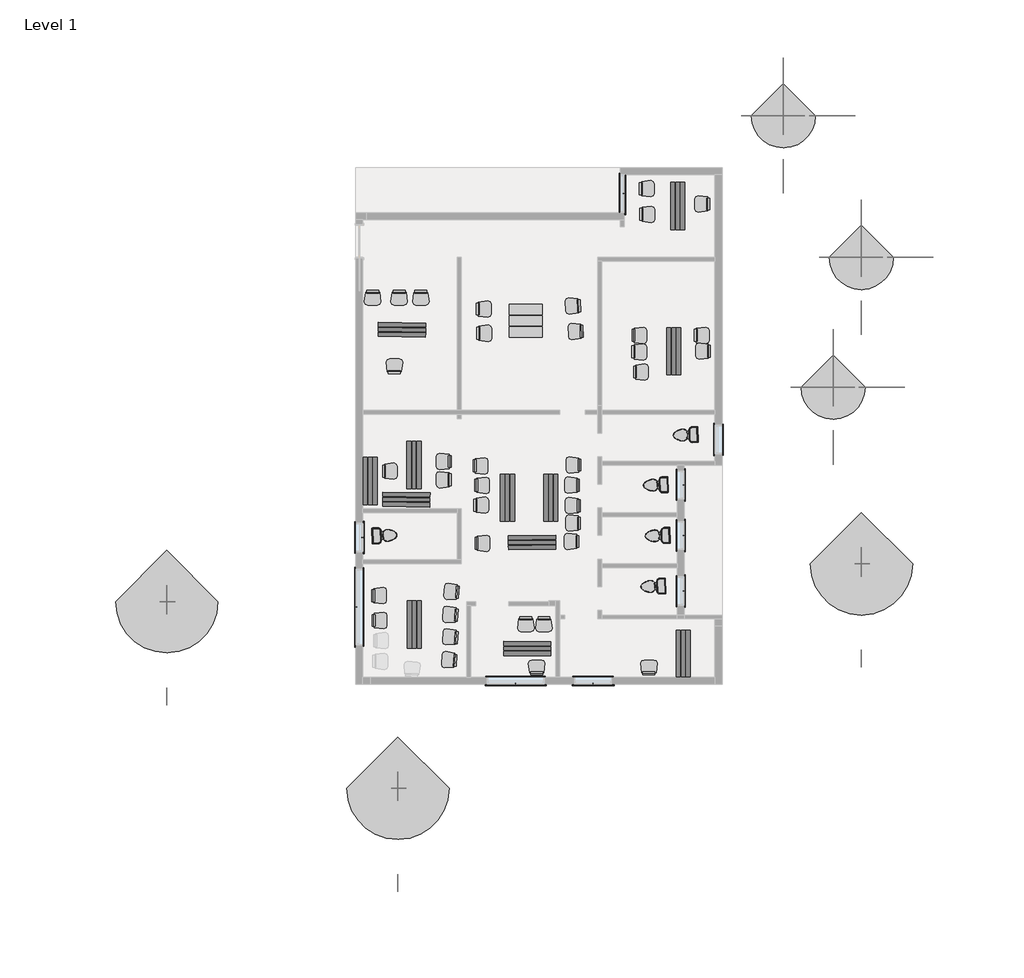
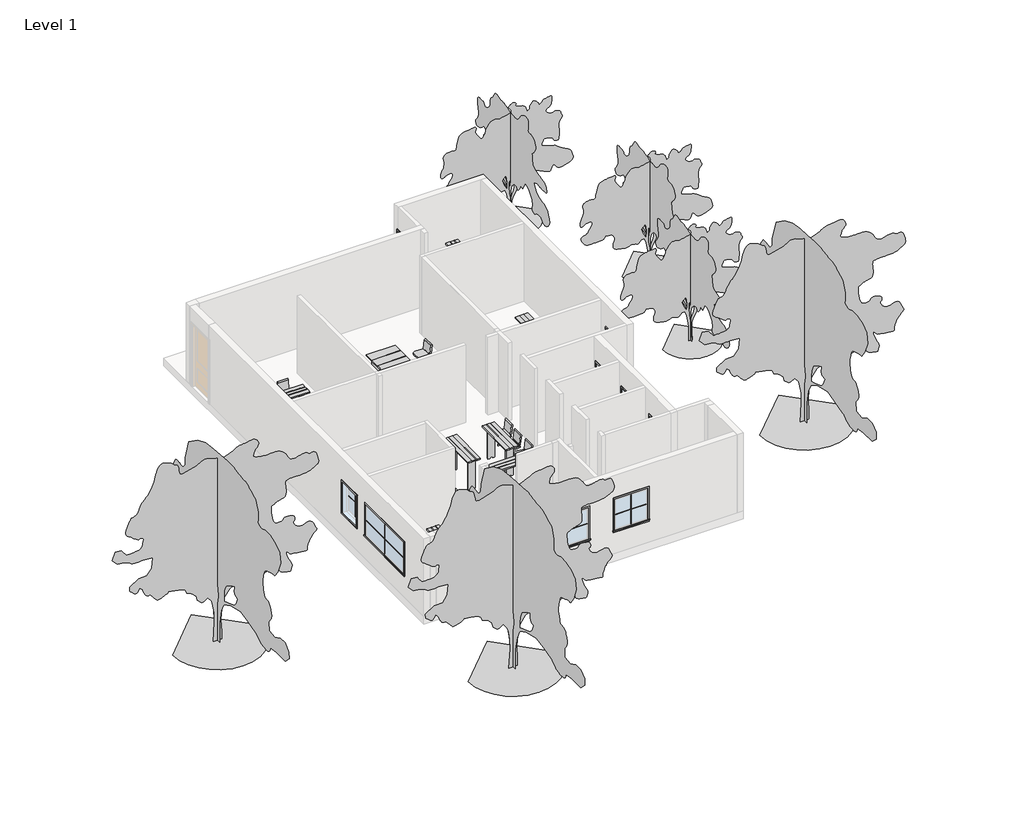
# One storey, part 2 of 2: 51 furniture elements, 27 proxies, 6 geographic elements, 5 flow terminals.
"""IFC4 building model written with IfcOpenShell, lengths in millimetres."""

from ifc_helpers import new_model, si_unit, origin, place, context, project, spatial, transform, mapped, element, save
from components import muntin_pattern_2x2_muntin_pattern_2x2_0b2f62cf, muntin_pattern_2x2_muntin_pattern_2x2_3e35e312, muntin_pattern_2x2_muntin_pattern_2x2_6be186e8, muntin_pattern_2x2_muntin_pattern_2x2_2dc59915, trim_window_exterior_flat_with_sill_e4b28ec3, trim_window_exterior_flat_with_sill_7cfdd449, trim_window_exterior_flat_with_sill_4ebd5beb, trim_window_exterior_flat_with_sill_02d88a07, trim_window_interior_flat_picture_frame_39ff4276, trim_window_interior_flat_picture_frame_f1e0b15b, trim_window_interior_flat_picture_frame_d03d3773, trim_window_interior_flat_picture_frame_03e64d7c, toilet_domestic_3d_toilet_domestic_3d_ba6479b0, toilet_domestic_3d_toilet_domestic_3d_30431060, furniture_f7008d8d, furniture_92cb3fd8, chair_desk_chair_desk_7ad88740, chair_desk_chair_desk_f6d25cbe, rpc_tree_deciduous_blue_berry_elder_15_a2d70376, rpc_tree_deciduous_hawthorn_25_a438f522

model = new_model("IFC4")

# Units and contexts
model_context = context("Model", 3, world=origin())
ifc_project = project(units=[si_unit("LENGTHUNIT", "METRE", prefix="MILLI")], contexts=[model_context])

# Site, building, storey
site = spatial("IfcSite", under=ifc_project)
building = spatial("IfcBuilding", under=site)
storey = spatial("IfcBuildingStorey", under=building, Name="Level 1", Elevation=0.0)

# Proxies
placement = place(None, origin())
muntin_pattern_2x2_muntin_pattern_2x2_shape = muntin_pattern_2x2_muntin_pattern_2x2_0b2f62cf(model_context)
element("IfcBuildingElementProxy", 1, Name="Muntin Pattern_2x2 : Muntin Pattern_2x2", ObjectType="Muntin Pattern_2x2 : Muntin Pattern_2x2", at=placement, inside=storey, context=model_context, shape_type="MappedRepresentation", body=[
    mapped(muntin_pattern_2x2_muntin_pattern_2x2_shape, transform((11852.275, 18726.15, 952.5), x_axis=(0.0, 1.0, 0.0), y_axis=(-1.0, 0.0, 0.0), z_axis=(0.0, 0.0, 1.0))),
])
element("IfcBuildingElementProxy", 2, Name="Muntin Pattern_2x2 : Muntin Pattern_2x2", ObjectType="Muntin Pattern_2x2 : Muntin Pattern_2x2", at=placement, inside=storey, context=model_context, shape_type="MappedRepresentation", body=[
    mapped(muntin_pattern_2x2_muntin_pattern_2x2_shape, transform((12861.925, 20186.0468811, 952.5), x_axis=(0.0, -1.0, 0.0), y_axis=(1.0, 0.0, 0.0), z_axis=(0.0, 0.0, 1.0))),
])
element("IfcBuildingElementProxy", 3, Name="Muntin Pattern_2x2 : Muntin Pattern_2x2", ObjectType="Muntin Pattern_2x2 : Muntin Pattern_2x2", at=placement, inside=storey, context=model_context, shape_type="MappedRepresentation", body=[
    mapped(muntin_pattern_2x2_muntin_pattern_2x2_shape, transform((1489.075, 17029.3631818, 952.5), x_axis=(0.0, 1.0, 0.0), y_axis=(-1.0, 0.0, 0.0), z_axis=(0.0, 0.0, 1.0))),
])
element("IfcBuildingElementProxy", 4, Name="Muntin Pattern_2x2 : Muntin Pattern_2x2", ObjectType="Muntin Pattern_2x2 : Muntin Pattern_2x2", at=placement, inside=storey, context=model_context, shape_type="MappedRepresentation", body=[
    mapped(muntin_pattern_2x2_muntin_pattern_2x2_shape, transform((11852.275, 15299.8267416, 952.5), x_axis=(0.0, 1.0, 0.0), y_axis=(-1.0, 0.0, 0.0), z_axis=(0.0, 0.0, 1.0))),
])
element("IfcBuildingElementProxy", 5, Name="Muntin Pattern_2x2 : Muntin Pattern_2x2", ObjectType="Muntin Pattern_2x2 : Muntin Pattern_2x2", at=placement, inside=storey, context=model_context, shape_type="MappedRepresentation", body=[
    mapped(muntin_pattern_2x2_muntin_pattern_2x2_shape, transform((11852.275, 17092.3067598, 952.5), x_axis=(0.0, 1.0, 0.0), y_axis=(-1.0, 0.0, 0.0), z_axis=(0.0, 0.0, 1.0))),
])
muntin_pattern_2x2_muntin_pattern_2x2_2_shape = muntin_pattern_2x2_muntin_pattern_2x2_3e35e312(model_context)
element("IfcBuildingElementProxy", 6, Name="Muntin Pattern_2x2 : Muntin Pattern_2x2", ObjectType="Muntin Pattern_2x2 : Muntin Pattern_2x2", at=placement, inside=storey, context=model_context, shape_type="MappedRepresentation", body=[
    mapped(muntin_pattern_2x2_muntin_pattern_2x2_2_shape, transform((9921.875, 28117.8, 952.5), x_axis=(0.0, 1.0, 0.0), y_axis=(-1.0, 0.0, 0.0), z_axis=(0.0, 0.0, 1.0))),
])
element("IfcBuildingElementProxy", 7, Name="Muntin Pattern_2x2 : Muntin Pattern_2x2", ObjectType="Muntin Pattern_2x2 : Muntin Pattern_2x2", at=placement, inside=storey, context=model_context, shape_type="MappedRepresentation", body=[
    mapped(muntin_pattern_2x2_muntin_pattern_2x2_2_shape, transform((8921.75, 12303.125, 952.5), x_axis=(1.0, 0.0, 0.0), y_axis=(0.0, 1.0, 0.0), z_axis=(0.0, 0.0, 1.0))),
])
muntin_pattern_2x2_muntin_pattern_2x2_3_shape = muntin_pattern_2x2_muntin_pattern_2x2_6be186e8(model_context)
element("IfcBuildingElementProxy", 8, Name="Muntin Pattern_2x2 : Muntin Pattern_2x2", ObjectType="Muntin Pattern_2x2 : Muntin Pattern_2x2", at=placement, inside=storey, context=model_context, shape_type="MappedRepresentation", body=[
    mapped(muntin_pattern_2x2_muntin_pattern_2x2_3_shape, transform((1279.525, 14783.4980131, 952.5), x_axis=(0.0, -1.0, 0.0), y_axis=(1.0, 0.0, 0.0), z_axis=(0.0, 0.0, 1.0))),
])
muntin_pattern_2x2_muntin_pattern_2x2_4_shape = muntin_pattern_2x2_muntin_pattern_2x2_2dc59915(model_context)
element("IfcBuildingElementProxy", 9, Name="Muntin Pattern_2x2 : Muntin Pattern_2x2", ObjectType="Muntin Pattern_2x2 : Muntin Pattern_2x2", at=placement, inside=storey, context=model_context, shape_type="MappedRepresentation", body=[
    mapped(muntin_pattern_2x2_muntin_pattern_2x2_4_shape, transform((6426.2, 12303.125, 952.5), x_axis=(1.0, 0.0, 0.0), y_axis=(0.0, 1.0, 0.0), z_axis=(0.0, 0.0, 1.0))),
])
trim_window_exterior_flat_with_sill_shape = trim_window_exterior_flat_with_sill_e4b28ec3(model_context)
element("IfcBuildingElementProxy", 10, Name="Trim-Window-Exterior-Flat : with Sill", ObjectType="Trim-Window-Exterior-Flat : with Sill", at=placement, inside=storey, context=model_context, shape_type="MappedRepresentation", body=[
    mapped(trim_window_exterior_flat_with_sill_shape, transform((11861.8, 18726.15, 2133.6), x_axis=(0.0, 1.0, 0.0), y_axis=(0.0, 0.0, 1.0), z_axis=(1.0, 0.0, 0.0))),
])
element("IfcBuildingElementProxy", 11, Name="Trim-Window-Exterior-Flat : with Sill", ObjectType="Trim-Window-Exterior-Flat : with Sill", at=placement, inside=storey, context=model_context, shape_type="MappedRepresentation", body=[
    mapped(trim_window_exterior_flat_with_sill_shape, transform((12852.4, 20186.0468811, 2133.6), x_axis=(0.0, -1.0, 0.0), y_axis=(0.0, 0.0, 1.0), z_axis=(-1.0, 0.0, 0.0))),
])
element("IfcBuildingElementProxy", 12, Name="Trim-Window-Exterior-Flat : with Sill", ObjectType="Trim-Window-Exterior-Flat : with Sill", at=placement, inside=storey, context=model_context, shape_type="MappedRepresentation", body=[
    mapped(trim_window_exterior_flat_with_sill_shape, transform((1498.6, 17029.3631818, 2133.6), x_axis=(0.0, 1.0, 0.0), y_axis=(0.0, 0.0, 1.0), z_axis=(1.0, 0.0, 0.0))),
])
element("IfcBuildingElementProxy", 13, Name="Trim-Window-Exterior-Flat : with Sill", ObjectType="Trim-Window-Exterior-Flat : with Sill", at=placement, inside=storey, context=model_context, shape_type="MappedRepresentation", body=[
    mapped(trim_window_exterior_flat_with_sill_shape, transform((11861.8, 15299.8267416, 2133.6), x_axis=(0.0, 1.0, 0.0), y_axis=(0.0, 0.0, 1.0), z_axis=(1.0, 0.0, 0.0))),
])
element("IfcBuildingElementProxy", 14, Name="Trim-Window-Exterior-Flat : with Sill", ObjectType="Trim-Window-Exterior-Flat : with Sill", at=placement, inside=storey, context=model_context, shape_type="MappedRepresentation", body=[
    mapped(trim_window_exterior_flat_with_sill_shape, transform((11861.8, 17092.3067598, 2133.6), x_axis=(0.0, 1.0, 0.0), y_axis=(0.0, 0.0, 1.0), z_axis=(1.0, 0.0, 0.0))),
])
trim_window_exterior_flat_with_sill_2_shape = trim_window_exterior_flat_with_sill_7cfdd449(model_context)
element("IfcBuildingElementProxy", 15, Name="Trim-Window-Exterior-Flat : with Sill", ObjectType="Trim-Window-Exterior-Flat : with Sill", at=placement, inside=storey, context=model_context, shape_type="MappedRepresentation", body=[
    mapped(trim_window_exterior_flat_with_sill_2_shape, transform((9931.4, 28117.8, 2133.6), x_axis=(0.0, 1.0, 0.0), y_axis=(0.0, 0.0, 1.0), z_axis=(1.0, 0.0, 0.0))),
])
element("IfcBuildingElementProxy", 16, Name="Trim-Window-Exterior-Flat : with Sill", ObjectType="Trim-Window-Exterior-Flat : with Sill", at=placement, inside=storey, context=model_context, shape_type="MappedRepresentation", body=[
    mapped(trim_window_exterior_flat_with_sill_2_shape, transform((8921.75, 12293.6, 2133.6), x_axis=(1.0, 0.0, 0.0), y_axis=(0.0, 0.0, 1.0), z_axis=(0.0, -1.0, 0.0))),
])
trim_window_exterior_flat_with_sill_3_shape = trim_window_exterior_flat_with_sill_4ebd5beb(model_context)
element("IfcBuildingElementProxy", 17, Name="Trim-Window-Exterior-Flat : with Sill", ObjectType="Trim-Window-Exterior-Flat : with Sill", at=placement, inside=storey, context=model_context, shape_type="MappedRepresentation", body=[
    mapped(trim_window_exterior_flat_with_sill_3_shape, transform((1270.0, 14783.4980131, 2133.6), x_axis=(0.0, -1.0, 0.0), y_axis=(0.0, 0.0, 1.0), z_axis=(-1.0, 0.0, 0.0))),
])
trim_window_exterior_flat_with_sill_4_shape = trim_window_exterior_flat_with_sill_02d88a07(model_context)
element("IfcBuildingElementProxy", 18, Name="Trim-Window-Exterior-Flat : with Sill", ObjectType="Trim-Window-Exterior-Flat : with Sill", at=placement, inside=storey, context=model_context, shape_type="MappedRepresentation", body=[
    mapped(trim_window_exterior_flat_with_sill_4_shape, transform((6426.2, 12293.6, 2133.6), x_axis=(1.0, 0.0, 0.0), y_axis=(0.0, 0.0, 1.0), z_axis=(0.0, -1.0, 0.0))),
])
trim_window_interior_flat_picture_frame_shape = trim_window_interior_flat_picture_frame_39ff4276(model_context)
element("IfcBuildingElementProxy", 19, Name="Trim-Window-Interior-Flat : Picture Frame", ObjectType="Trim-Window-Interior-Flat : Picture Frame", at=placement, inside=storey, context=model_context, shape_type="MappedRepresentation", body=[
    mapped(trim_window_interior_flat_picture_frame_shape, transform((11633.2, 18726.15, 2133.6), x_axis=(0.0, -1.0, 0.0), y_axis=(0.0, 0.0, 1.0), z_axis=(-1.0, 0.0, 0.0))),
])
element("IfcBuildingElementProxy", 20, Name="Trim-Window-Interior-Flat : Picture Frame", ObjectType="Trim-Window-Interior-Flat : Picture Frame", at=placement, inside=storey, context=model_context, shape_type="MappedRepresentation", body=[
    mapped(trim_window_interior_flat_picture_frame_shape, transform((13081.0, 20186.0468811, 2133.6), x_axis=(0.0, 1.0, 0.0), y_axis=(0.0, 0.0, 1.0), z_axis=(1.0, 0.0, 0.0))),
])
element("IfcBuildingElementProxy", 21, Name="Trim-Window-Interior-Flat : Picture Frame", ObjectType="Trim-Window-Interior-Flat : Picture Frame", at=placement, inside=storey, context=model_context, shape_type="MappedRepresentation", body=[
    mapped(trim_window_interior_flat_picture_frame_shape, transform((1270.0, 17029.3631818, 2133.6), x_axis=(0.0, -1.0, 0.0), y_axis=(0.0, 0.0, 1.0), z_axis=(-1.0, 0.0, 0.0))),
])
element("IfcBuildingElementProxy", 22, Name="Trim-Window-Interior-Flat : Picture Frame", ObjectType="Trim-Window-Interior-Flat : Picture Frame", at=placement, inside=storey, context=model_context, shape_type="MappedRepresentation", body=[
    mapped(trim_window_interior_flat_picture_frame_shape, transform((11633.2, 15299.8267416, 2133.6), x_axis=(0.0, -1.0, 0.0), y_axis=(0.0, 0.0, 1.0), z_axis=(-1.0, 0.0, 0.0))),
])
element("IfcBuildingElementProxy", 23, Name="Trim-Window-Interior-Flat : Picture Frame", ObjectType="Trim-Window-Interior-Flat : Picture Frame", at=placement, inside=storey, context=model_context, shape_type="MappedRepresentation", body=[
    mapped(trim_window_interior_flat_picture_frame_shape, transform((11633.2, 17092.3067598, 2133.6), x_axis=(0.0, -1.0, 0.0), y_axis=(0.0, 0.0, 1.0), z_axis=(-1.0, 0.0, 0.0))),
])
trim_window_interior_flat_picture_frame_2_shape = trim_window_interior_flat_picture_frame_f1e0b15b(model_context)
element("IfcBuildingElementProxy", 24, Name="Trim-Window-Interior-Flat : Picture Frame", ObjectType="Trim-Window-Interior-Flat : Picture Frame", at=placement, inside=storey, context=model_context, shape_type="MappedRepresentation", body=[
    mapped(trim_window_interior_flat_picture_frame_2_shape, transform((9804.4, 28117.8, 2133.6), x_axis=(0.0, -1.0, 0.0), y_axis=(0.0, 0.0, 1.0), z_axis=(-1.0, 0.0, 0.0))),
])
element("IfcBuildingElementProxy", 25, Name="Trim-Window-Interior-Flat : Picture Frame", ObjectType="Trim-Window-Interior-Flat : Picture Frame", at=placement, inside=storey, context=model_context, shape_type="MappedRepresentation", body=[
    mapped(trim_window_interior_flat_picture_frame_2_shape, transform((8921.75, 12522.2, 2133.6), x_axis=(-1.0, 0.0, 0.0), y_axis=(0.0, 0.0, 1.0), z_axis=(0.0, 1.0, 0.0))),
])
trim_window_interior_flat_picture_frame_3_shape = trim_window_interior_flat_picture_frame_d03d3773(model_context)
element("IfcBuildingElementProxy", 26, Name="Trim-Window-Interior-Flat : Picture Frame", ObjectType="Trim-Window-Interior-Flat : Picture Frame", at=placement, inside=storey, context=model_context, shape_type="MappedRepresentation", body=[
    mapped(trim_window_interior_flat_picture_frame_3_shape, transform((1498.6, 14783.4980131, 2133.6), x_axis=(0.0, 1.0, 0.0), y_axis=(0.0, 0.0, 1.0), z_axis=(1.0, 0.0, 0.0))),
])
trim_window_interior_flat_picture_frame_4_shape = trim_window_interior_flat_picture_frame_03e64d7c(model_context)
element("IfcBuildingElementProxy", 27, Name="Trim-Window-Interior-Flat : Picture Frame", ObjectType="Trim-Window-Interior-Flat : Picture Frame", at=placement, inside=storey, context=model_context, shape_type="MappedRepresentation", body=[
    mapped(trim_window_interior_flat_picture_frame_4_shape, transform((6426.2, 12522.2, 2133.6), x_axis=(-1.0, 0.0, 0.0), y_axis=(0.0, 0.0, 1.0), z_axis=(0.0, 1.0, 0.0))),
])

# Flow terminals
toilet_domestic_3d_toilet_domestic_3d_shape = toilet_domestic_3d_toilet_domestic_3d_ba6479b0(model_context)
toilet_domestic_3d_toilet_domestic_3d_2_shape = toilet_domestic_3d_toilet_domestic_3d_30431060(model_context)
element("IfcFlowTerminal", 28, ObjectType="Toilet-Domestic-3D : Toilet-Domestic-3D", at=placement, inside=storey, context=model_context, shape_type="MappedRepresentation", body=[
    mapped(toilet_domestic_3d_toilet_domestic_3d_shape, transform((11812.081271, 20333.332001, 0.0), x_axis=(0.0355411275689283, -0.9993682145491367, 0.0), y_axis=(0.9993682145491367, 0.0355411275689283, 0.0), z_axis=(0.0, 0.0, 1.0))),
    mapped(toilet_domestic_3d_toilet_domestic_3d_2_shape, transform((11812.081271, 20333.332001, 0.0), x_axis=(0.0355411275689283, -0.9993682145491367, 0.0), y_axis=(0.9993682145491367, 0.0355411275689283, 0.0), z_axis=(0.0, 0.0, 1.0))),
])
element("IfcFlowTerminal", 29, ObjectType="Toilet-Domestic-3D : Toilet-Domestic-3D", at=placement, inside=storey, context=model_context, shape_type="MappedRepresentation", body=[
    mapped(toilet_domestic_3d_toilet_domestic_3d_shape, transform((10850.8877462, 18719.2515392, 0.0), x_axis=(0.03554112756892187, -0.9993682145491369, 0.0), y_axis=(0.9993682145491369, 0.03554112756892187, 0.0), z_axis=(0.0, 0.0, 1.0))),
    mapped(toilet_domestic_3d_toilet_domestic_3d_2_shape, transform((10850.8877462, 18719.2515392, 0.0), x_axis=(0.03554112756892187, -0.9993682145491369, 0.0), y_axis=(0.9993682145491369, 0.03554112756892187, 0.0), z_axis=(0.0, 0.0, 1.0))),
])
element("IfcFlowTerminal", 30, ObjectType="Toilet-Domestic-3D : Toilet-Domestic-3D", at=placement, inside=storey, context=model_context, shape_type="MappedRepresentation", body=[
    mapped(toilet_domestic_3d_toilet_domestic_3d_shape, transform((10908.9901447, 17085.4910432, 0.0), x_axis=(0.03554112756892187, -0.9993682145491369, 0.0), y_axis=(0.9993682145491369, 0.03554112756892187, 0.0), z_axis=(0.0, 0.0, 1.0))),
    mapped(toilet_domestic_3d_toilet_domestic_3d_2_shape, transform((10908.9901447, 17085.4910432, 0.0), x_axis=(0.03554112756892187, -0.9993682145491369, 0.0), y_axis=(0.9993682145491369, 0.03554112756892187, 0.0), z_axis=(0.0, 0.0, 1.0))),
])
element("IfcFlowTerminal", 31, ObjectType="Toilet-Domestic-3D : Toilet-Domestic-3D", at=placement, inside=storey, context=model_context, shape_type="MappedRepresentation", body=[
    mapped(toilet_domestic_3d_toilet_domestic_3d_shape, transform((10770.2616437, 15450.0084658, 0.0), x_axis=(0.03554112756892187, -0.9993682145491369, 0.0), y_axis=(0.9993682145491369, 0.03554112756892187, 0.0), z_axis=(0.0, 0.0, 1.0))),
    mapped(toilet_domestic_3d_toilet_domestic_3d_2_shape, transform((10770.2616437, 15450.0084658, 0.0), x_axis=(0.03554112756892187, -0.9993682145491369, 0.0), y_axis=(0.9993682145491369, 0.03554112756892187, 0.0), z_axis=(0.0, 0.0, 1.0))),
])
element("IfcFlowTerminal", 32, ObjectType="Toilet-Domestic-3D : Toilet-Domestic-3D", at=placement, inside=storey, context=model_context, shape_type="MappedRepresentation", body=[
    mapped(toilet_domestic_3d_toilet_domestic_3d_shape, transform((2292.7062712, 17095.9305022, 0.0), x_axis=(-0.03572734203544766, 0.9993615747221234, 0.0), y_axis=(-0.9993615747221234, -0.03572734203544766, 0.0), z_axis=(0.0, 0.0, 1.0))),
    mapped(toilet_domestic_3d_toilet_domestic_3d_2_shape, transform((2292.7062712, 17095.9305022, 0.0), x_axis=(-0.03572734203544766, 0.9993615747221234, 0.0), y_axis=(-0.9993615747221234, -0.03572734203544766, 0.0), z_axis=(0.0, 0.0, 1.0))),
])

# Furniture
furniture_shape = furniture_f7008d8d(model_context)
element("IfcFurniture", 33, ObjectType="Bench-Locker Room : 48\" x 18\" x 14\"", at=placement, inside=storey, context=model_context, shape_type="MappedRepresentation", body=[
    mapped(furniture_shape, transform((2974.0575649, 14379.3147541, 0.0), x_axis=(0.0, 1.0, 0.0), y_axis=(-1.0, 0.0, 0.0), z_axis=(0.0, 0.0, 1.0))),
])
element("IfcFurniture", 34, ObjectType="Bench-Locker Room : 48\" x 18\" x 14\"", at=placement, inside=storey, context=model_context, shape_type="MappedRepresentation", body=[
    mapped(furniture_shape, transform((2917.3364211, 23908.3455859, 0.0), x_axis=(0.9998480894786371, -0.017429801086626003, 0.0), y_axis=(0.017429801086626003, 0.9998480894786371, 0.0), z_axis=(0.0, 0.0, 1.0))),
])
element("IfcFurniture", 35, ObjectType="Bench-Locker Room : 48\" x 18\" x 14\"", at=placement, inside=storey, context=model_context, shape_type="MappedRepresentation", body=[
    mapped(furniture_shape, transform((11830.2076457, 27568.7581913, 0.0), x_axis=(0.0, -1.0, 0.0), y_axis=(1.0, 0.0, 0.0), z_axis=(0.0, 0.0, 1.0))),
])
element("IfcFurniture", 36, ObjectType="Bench-Locker Room : 48\" x 18\" x 14\"", at=placement, inside=storey, context=model_context, shape_type="MappedRepresentation", body=[
    mapped(furniture_shape, transform((11704.0646955, 22884.2865861, 0.0), x_axis=(0.0, -1.0, 0.0), y_axis=(1.0, 0.0, 0.0), z_axis=(0.0, 0.0, 1.0))),
])
element("IfcFurniture", 37, ObjectType="Bench-Locker Room : 48\" x 18\" x 14\"", at=placement, inside=storey, context=model_context, shape_type="MappedRepresentation", body=[
    mapped(furniture_shape, transform((5979.6841277, 18462.9611479, 0.0), x_axis=(0.0, 1.0, 0.0), y_axis=(-1.0, 0.0, 0.0), z_axis=(0.0, 0.0, 1.0))),
])
element("IfcFurniture", 38, ObjectType="Bench-Locker Room : 48\" x 18\" x 14\"", at=placement, inside=storey, context=model_context, shape_type="MappedRepresentation", body=[
    mapped(furniture_shape, transform((6801.6796201, 16686.4490944, 0.0), x_axis=(-0.9999200930744279, -0.012641497776273655, 0.0), y_axis=(0.012641497776273655, -0.9999200930744279, 0.0), z_axis=(0.0, 0.0, 1.0))),
])
element("IfcFurniture", 39, ObjectType="Bench-Locker Room : 48\" x 18\" x 14\"", at=placement, inside=storey, context=model_context, shape_type="MappedRepresentation", body=[
    mapped(furniture_shape, transform((1553.7196201, 19010.7185302, 0.0), x_axis=(0.0, 1.0, 0.0), y_axis=(-1.0, 0.0, 0.0), z_axis=(0.0, 0.0, 1.0))),
])
element("IfcFurniture", 40, ObjectType="Bench-Locker Room : 48\" x 18\" x 14\"", at=placement, inside=storey, context=model_context, shape_type="MappedRepresentation", body=[
    mapped(furniture_shape, transform((12008.8646955, 13125.8549349, 0.0), x_axis=(0.0, -1.0, 0.0), y_axis=(1.0, 0.0, 0.0), z_axis=(0.0, 0.0, 1.0))),
])
element("IfcFurniture", 41, ObjectType="Bench-Locker Room : 48\" x 18\" x 14\"", at=placement, inside=storey, context=model_context, shape_type="MappedRepresentation", body=[
    mapped(furniture_shape, transform((6640.7852173, 13265.3501596, 0.0), x_axis=(-0.9999884249581985, 0.004811439454202483, 0.0), y_axis=(-0.004811439454202483, -0.9999884249581985, 0.0), z_axis=(0.0, 0.0, 1.0))),
])
element("IfcFurniture", 42, ObjectType="Bench-Locker Room : 48\" x 18\" x 14\"", at=placement, inside=storey, context=model_context, shape_type="MappedRepresentation", body=[
    mapped(furniture_shape, transform((3055.5684722, 18429.963506, 0.0), x_axis=(0.9998480894786371, -0.017429801086626003, 0.0), y_axis=(0.017429801086626003, 0.9998480894786371, 0.0), z_axis=(0.0, 0.0, 1.0))),
])
element("IfcFurniture", 43, ObjectType="Bench-Locker Room : 48\" x 18\" x 14\"", at=placement, inside=storey, context=model_context, shape_type="MappedRepresentation", body=[
    mapped(furniture_shape, transform((7381.3152378, 18462.9611479, 0.0), x_axis=(0.0, 1.0, 0.0), y_axis=(-1.0, 0.0, 0.0), z_axis=(0.0, 0.0, 1.0))),
])
element("IfcFurniture", 44, ObjectType="Bench-Locker Room : 48\" x 18\" x 14\"", at=placement, inside=storey, context=model_context, shape_type="MappedRepresentation", body=[
    mapped(furniture_shape, transform((2964.6454164, 19518.8936677, 0.0), x_axis=(0.0, 1.0, 0.0), y_axis=(-1.0, 0.0, 0.0), z_axis=(0.0, 0.0, 1.0))),
])
furniture_2_shape = furniture_92cb3fd8(model_context)
element("IfcFurniture", 45, ObjectType="Bench-Locker Room : 48\" x 18\" x 18\"", at=placement, inside=storey, context=model_context, shape_type="MappedRepresentation", body=[
    mapped(furniture_2_shape, transform((6908.1087006, 24204.188932, 0.0), x_axis=(1.0, 0.0, 0.0), y_axis=(0.0, 1.0, 0.0), z_axis=(0.0, 0.0, 1.0))),
])
chair_desk_chair_desk_shape = chair_desk_chair_desk_7ad88740(model_context)
element("IfcFurniture", 46, ObjectType="Chair-Desk : Chair-Desk", at=placement, inside=storey, context=model_context, shape_type="MappedRepresentation", body=[
    mapped(chair_desk_chair_desk_shape, transform((8397.3520149, 16903.7, 0.0), x_axis=(0.0, 1.0, 0.0), y_axis=(-1.0, 0.0, 0.0), z_axis=(0.0, 0.0, 1.0))),
])
element("IfcFurniture", 47, ObjectType="Chair-Desk : Chair-Desk", at=placement, inside=storey, context=model_context, shape_type="MappedRepresentation", body=[
    mapped(chair_desk_chair_desk_shape, transform((8444.7345696, 17494.2878949, 0.0), x_axis=(0.0, 1.0, 0.0), y_axis=(-1.0, 0.0, 0.0), z_axis=(0.0, 0.0, 1.0))),
])
element("IfcFurniture", 48, ObjectType="Chair-Desk : Chair-Desk", at=placement, inside=storey, context=model_context, shape_type="MappedRepresentation", body=[
    mapped(chair_desk_chair_desk_shape, transform((8438.3933452, 18054.041753, 0.0), x_axis=(0.0, 1.0, 0.0), y_axis=(-1.0, 0.0, 0.0), z_axis=(0.0, 0.0, 1.0))),
])
element("IfcFurniture", 49, ObjectType="Chair-Desk : Chair-Desk", at=placement, inside=storey, context=model_context, shape_type="MappedRepresentation", body=[
    mapped(chair_desk_chair_desk_shape, transform((4278.1176051, 19481.8, 0.0), x_axis=(0.0, 1.0, 0.0), y_axis=(-1.0, 0.0, 0.0), z_axis=(0.0, 0.0, 1.0))),
])
element("IfcFurniture", 50, ObjectType="Chair-Desk : Chair-Desk", at=placement, inside=storey, context=model_context, shape_type="MappedRepresentation", body=[
    mapped(chair_desk_chair_desk_shape, transform((4275.5800785, 18890.7524599, 0.0), x_axis=(0.0, 1.0, 0.0), y_axis=(-1.0, 0.0, 0.0), z_axis=(0.0, 0.0, 1.0))),
])
element("IfcFurniture", 51, ObjectType="Chair-Desk : Chair-Desk", at=placement, inside=storey, context=model_context, shape_type="MappedRepresentation", body=[
    mapped(chair_desk_chair_desk_shape, transform((8410.2496775, 18715.0954423, 0.0), x_axis=(0.0, 1.0, 0.0), y_axis=(-1.0, 0.0, 0.0), z_axis=(0.0, 0.0, 1.0))),
])
element("IfcFurniture", 52, ObjectType="Chair-Desk : Chair-Desk", at=placement, inside=storey, context=model_context, shape_type="MappedRepresentation", body=[
    mapped(chair_desk_chair_desk_shape, transform((2197.4822905, 19168.4618696, 0.0), x_axis=(0.0, -1.0, 0.0), y_axis=(1.0, 0.0, 0.0), z_axis=(0.0, 0.0, 1.0))),
])
element("IfcFurniture", 53, ObjectType="Chair-Desk : Chair-Desk", at=placement, inside=storey, context=model_context, shape_type="MappedRepresentation", body=[
    mapped(chair_desk_chair_desk_shape, transform((5125.0631491, 19335.7449431, 0.0), x_axis=(0.0, -1.0, 0.0), y_axis=(1.0, 0.0, 0.0), z_axis=(0.0, 0.0, 1.0))),
])
element("IfcFurniture", 54, ObjectType="Chair-Desk : Chair-Desk", at=placement, inside=storey, context=model_context, shape_type="MappedRepresentation", body=[
    mapped(chair_desk_chair_desk_shape, transform((5173.5648431, 18713.4149099, 0.0), x_axis=(0.0, -1.0, 0.0), y_axis=(1.0, 0.0, 0.0), z_axis=(0.0, 0.0, 1.0))),
])
element("IfcFurniture", 55, ObjectType="Chair-Desk : Chair-Desk", at=placement, inside=storey, context=model_context, shape_type="MappedRepresentation", body=[
    mapped(chair_desk_chair_desk_shape, transform((5146.5403146, 18072.1432431, 0.0), x_axis=(0.0, -1.0, 0.0), y_axis=(1.0, 0.0, 0.0), z_axis=(0.0, 0.0, 1.0))),
])
element("IfcFurniture", 56, ObjectType="Chair-Desk : Chair-Desk", at=placement, inside=storey, context=model_context, shape_type="MappedRepresentation", body=[
    mapped(chair_desk_chair_desk_shape, transform((12256.0694835, 23545.9420373, 0.0), x_axis=(0.0, -1.0, 0.0), y_axis=(1.0, 0.0, 0.0), z_axis=(0.0, 0.0, 1.0))),
])
element("IfcFurniture", 57, ObjectType="Chair-Desk : Chair-Desk", at=placement, inside=storey, context=model_context, shape_type="MappedRepresentation", body=[
    mapped(chair_desk_chair_desk_shape, transform((5187.5816449, 16839.2593518, 0.0), x_axis=(0.0, -1.0, 0.0), y_axis=(1.0, 0.0, 0.0), z_axis=(0.0, 0.0, 1.0))),
])
element("IfcFurniture", 58, ObjectType="Chair-Desk : Chair-Desk", at=placement, inside=storey, context=model_context, shape_type="MappedRepresentation", body=[
    mapped(chair_desk_chair_desk_shape, transform((1811.6036816, 24933.2977629, 0.0), x_axis=(-1.0, 0.0, 0.0), y_axis=(0.0, -1.0, 0.0), z_axis=(0.0, 0.0, 1.0))),
])
element("IfcFurniture", 59, ObjectType="Chair-Desk : Chair-Desk", at=placement, inside=storey, context=model_context, shape_type="MappedRepresentation", body=[
    mapped(chair_desk_chair_desk_shape, transform((2665.4699803, 24933.2977629, 0.0), x_axis=(-1.0, 0.0, 0.0), y_axis=(0.0, -1.0, 0.0), z_axis=(0.0, 0.0, 1.0))),
])
element("IfcFurniture", 60, ObjectType="Chair-Desk : Chair-Desk", at=placement, inside=storey, context=model_context, shape_type="MappedRepresentation", body=[
    mapped(chair_desk_chair_desk_shape, transform((3366.8585021, 24931.0160368, 0.0), x_axis=(-1.0, 0.0, 0.0), y_axis=(0.0, -1.0, 0.0), z_axis=(0.0, 0.0, 1.0))),
])
element("IfcFurniture", 61, ObjectType="Chair-Desk : Chair-Desk", at=placement, inside=storey, context=model_context, shape_type="MappedRepresentation", body=[
    mapped(chair_desk_chair_desk_shape, transform((2513.070397, 22382.7591079, 0.0), x_axis=(1.0, 0.0, 0.0), y_axis=(0.0, 1.0, 0.0), z_axis=(0.0, 0.0, 1.0))),
])
element("IfcFurniture", 62, ObjectType="Chair-Desk : Chair-Desk", at=placement, inside=storey, context=model_context, shape_type="MappedRepresentation", body=[
    mapped(chair_desk_chair_desk_shape, transform((5225.3868389, 24395.7359018, 0.0), x_axis=(0.0, -1.0, 0.0), y_axis=(1.0, 0.0, 0.0), z_axis=(0.0, 0.0, 1.0))),
])
element("IfcFurniture", 63, ObjectType="Chair-Desk : Chair-Desk", at=placement, inside=storey, context=model_context, shape_type="MappedRepresentation", body=[
    mapped(chair_desk_chair_desk_shape, transform((8444.9300859, 24505.9413596, 0.0), x_axis=(-0.044220820600650974, 0.999021781056552, 0.0), y_axis=(-0.999021781056552, -0.044220820600650974, 0.0), z_axis=(0.0, 0.0, 1.0))),
])
element("IfcFurniture", 64, ObjectType="Chair-Desk : Chair-Desk", at=placement, inside=storey, context=model_context, shape_type="MappedRepresentation", body=[
    mapped(chair_desk_chair_desk_shape, transform((8532.6046479, 23683.7956886, 0.0), x_axis=(-0.023562510229805312, 0.9997223655153816, 0.0), y_axis=(-0.9997223655153816, -0.023562510229805312, 0.0), z_axis=(0.0, 0.0, 1.0))),
])
element("IfcFurniture", 65, ObjectType="Chair-Desk : Chair-Desk", at=placement, inside=storey, context=model_context, shape_type="MappedRepresentation", body=[
    mapped(chair_desk_chair_desk_shape, transform((12640.9499414, 23039.6013401, 0.0), x_axis=(0.0, 1.0, 0.0), y_axis=(-1.0, 0.0, 0.0), z_axis=(0.0, 0.0, 1.0))),
])
element("IfcFurniture", 66, ObjectType="Chair-Desk : Chair-Desk", at=placement, inside=storey, context=model_context, shape_type="MappedRepresentation", body=[
    mapped(chair_desk_chair_desk_shape, transform((10250.8028077, 23545.9420373, 0.0), x_axis=(0.0, -1.0, 0.0), y_axis=(1.0, 0.0, 0.0), z_axis=(0.0, 0.0, 1.0))),
])
element("IfcFurniture", 67, ObjectType="Chair-Desk : Chair-Desk", at=placement, inside=storey, context=model_context, shape_type="MappedRepresentation", body=[
    mapped(chair_desk_chair_desk_shape, transform((5241.9810911, 23616.9664056, 0.0), x_axis=(0.0, -1.0, 0.0), y_axis=(1.0, 0.0, 0.0), z_axis=(0.0, 0.0, 1.0))),
])
element("IfcFurniture", 68, ObjectType="Chair-Desk : Chair-Desk", at=placement, inside=storey, context=model_context, shape_type="MappedRepresentation", body=[
    mapped(chair_desk_chair_desk_shape, transform((10244.4615833, 23011.5881792, 0.0), x_axis=(0.0, -1.0, 0.0), y_axis=(1.0, 0.0, 0.0), z_axis=(0.0, 0.0, 1.0))),
])
element("IfcFurniture", 69, ObjectType="Chair-Desk : Chair-Desk", at=placement, inside=storey, context=model_context, shape_type="MappedRepresentation", body=[
    mapped(chair_desk_chair_desk_shape, transform((10292.9632773, 22363.8581459, 0.0), x_axis=(0.0, -1.0, 0.0), y_axis=(1.0, 0.0, 0.0), z_axis=(0.0, 0.0, 1.0))),
])
element("IfcFurniture", 70, ObjectType="Chair-Desk : Chair-Desk", at=placement, inside=storey, context=model_context, shape_type="MappedRepresentation", body=[
    mapped(chair_desk_chair_desk_shape, transform((1852.1687315, 15153.7242893, 0.0), x_axis=(0.0, -1.0, 0.0), y_axis=(1.0, 0.0, 0.0), z_axis=(0.0, 0.0, 1.0))),
])
element("IfcFurniture", 71, ObjectType="Chair-Desk : Chair-Desk", at=placement, inside=storey, context=model_context, shape_type="MappedRepresentation", body=[
    mapped(chair_desk_chair_desk_shape, transform((1867.6438444, 14349.5547931, 0.0), x_axis=(0.0, -1.0, 0.0), y_axis=(1.0, 0.0, 0.0), z_axis=(0.0, 0.0, 1.0))),
])
element("IfcFurniture", 72, ObjectType="Chair-Desk : Chair-Desk", at=placement, inside=storey, context=model_context, shape_type="MappedRepresentation", body=[
    mapped(chair_desk_chair_desk_shape, transform((4487.5834312, 14528.6192567, 0.0), x_axis=(0.07165305639653614, 0.9974296163183821, 0.0), y_axis=(-0.9974296163183821, 0.07165305639653614, 0.0), z_axis=(0.0, 0.0, 1.0))),
])
element("IfcFurniture", 73, ObjectType="Chair-Desk : Chair-Desk", at=placement, inside=storey, context=model_context, shape_type="MappedRepresentation", body=[
    mapped(chair_desk_chair_desk_shape, transform((4526.0991963, 15272.2986726, 0.0), x_axis=(0.07165305639653659, 0.997429616318382, 0.0), y_axis=(-0.997429616318382, 0.07165305639653659, 0.0), z_axis=(0.0, 0.0, 1.0))),
])
element("IfcFurniture", 74, ObjectType="Chair-Desk : Chair-Desk", at=placement, inside=storey, context=model_context, shape_type="MappedRepresentation", body=[
    mapped(chair_desk_chair_desk_shape, transform((4486.7693024, 13806.5500014, 0.0), x_axis=(0.07165305639653659, 0.997429616318382, 0.0), y_axis=(-0.997429616318382, 0.07165305639653659, 0.0), z_axis=(0.0, 0.0, 1.0))),
])
element("IfcFurniture", 75, ObjectType="Chair-Desk : Chair-Desk", at=placement, inside=storey, context=model_context, shape_type="MappedRepresentation", body=[
    mapped(chair_desk_chair_desk_shape, transform((4449.884969, 13067.78431, 0.0), x_axis=(0.07165305639653659, 0.997429616318382, 0.0), y_axis=(-0.997429616318382, 0.07165305639653659, 0.0), z_axis=(0.0, 0.0, 1.0))),
])
element("IfcFurniture", 76, ObjectType="Chair-Desk : Chair-Desk", at=placement, inside=storey, context=model_context, shape_type="MappedRepresentation", body=[
    mapped(chair_desk_chair_desk_shape, transform((6753.5114782, 14401.8, 0.0), x_axis=(-1.0, 0.0, 0.0), y_axis=(0.0, -1.0, 0.0), z_axis=(0.0, 0.0, 1.0))),
])
element("IfcFurniture", 77, ObjectType="Chair-Desk : Chair-Desk", at=placement, inside=storey, context=model_context, shape_type="MappedRepresentation", body=[
    mapped(chair_desk_chair_desk_shape, transform((7334.612421, 14399.4975355, 0.0), x_axis=(-1.0, 0.0, 0.0), y_axis=(0.0, -1.0, 0.0), z_axis=(0.0, 0.0, 1.0))),
])
element("IfcFurniture", 78, ObjectType="Chair-Desk : Chair-Desk", at=placement, inside=storey, context=model_context, shape_type="MappedRepresentation", body=[
    mapped(chair_desk_chair_desk_shape, transform((7103.213807, 12671.569689, 0.0), x_axis=(1.0, 0.0, 0.0), y_axis=(0.0, 1.0, 0.0), z_axis=(0.0, 0.0, 1.0))),
])
element("IfcFurniture", 79, ObjectType="Chair-Desk : Chair-Desk", at=placement, inside=storey, context=model_context, shape_type="MappedRepresentation", body=[
    mapped(chair_desk_chair_desk_shape, transform((10724.1296667, 12671.569689, 0.0), x_axis=(1.0, 0.0, 0.0), y_axis=(0.0, 1.0, 0.0), z_axis=(0.0, 0.0, 1.0))),
])
element("IfcFurniture", 80, ObjectType="Chair-Desk : Chair-Desk", at=placement, inside=storey, context=model_context, shape_type="MappedRepresentation", body=[
    mapped(chair_desk_chair_desk_shape, transform((10500.7429705, 27450.4869956, 0.0), x_axis=(0.0, -1.0, 0.0), y_axis=(1.0, 0.0, 0.0), z_axis=(0.0, 0.0, 1.0))),
])
element("IfcFurniture", 81, ObjectType="Chair-Desk : Chair-Desk", at=placement, inside=storey, context=model_context, shape_type="MappedRepresentation", body=[
    mapped(chair_desk_chair_desk_shape, transform((10485.2678575, 28280.0564918, 0.0), x_axis=(0.0, -1.0, 0.0), y_axis=(1.0, 0.0, 0.0), z_axis=(0.0, 0.0, 1.0))),
])
element("IfcFurniture", 82, ObjectType="Chair-Desk : Chair-Desk", at=placement, inside=storey, context=model_context, shape_type="MappedRepresentation", body=[
    mapped(chair_desk_chair_desk_shape, transform((12613.0097635, 27788.8751116, 0.0), x_axis=(0.0, 1.0, 0.0), y_axis=(-1.0, 0.0, 0.0), z_axis=(0.0, 0.0, 1.0))),
])
chair_desk_chair_desk_2_shape = chair_desk_chair_desk_f6d25cbe(model_context)
element("IfcFurniture", 83, ObjectType="Chair-Desk : Chair-Desk", at=placement, inside=storey, context=model_context, shape_type="MappedRepresentation", body=[
    mapped(chair_desk_chair_desk_2_shape, transform((8458.7513715, 19364.4392537, 0.0), x_axis=(0.0, -1.0, 0.0), y_axis=(1.0, 0.0, 0.0), z_axis=(0.0, 0.0, 1.0))),
])

# Geographic elements
rpc_tree_deciduous_blue_berry_elder_15_shape = rpc_tree_deciduous_blue_berry_elder_15_a2d70376(model_context)
element("IfcGeographicElement", 84, ObjectType="RPC Tree - Deciduous : Blue Berry Elder - 15'", at=placement, inside=storey, context=model_context, shape_type="MappedRepresentation", body=[
    mapped(rpc_tree_deciduous_blue_berry_elder_15_shape, transform((15062.2, 30632.4, -406.4), x_axis=(1.0, 0.0, 0.0), y_axis=(0.0, 1.0, 0.0), z_axis=(0.0, 0.0, 1.0))),
])
element("IfcGeographicElement", 85, ObjectType="RPC Tree - Deciduous : Blue Berry Elder - 15'", at=placement, inside=storey, context=model_context, shape_type="MappedRepresentation", body=[
    mapped(rpc_tree_deciduous_blue_berry_elder_15_shape, transform((17576.8, 26060.4, -406.4), x_axis=(1.0, 0.0, 0.0), y_axis=(0.0, 1.0, 0.0), z_axis=(0.0, 0.0, 1.0))),
])
element("IfcGeographicElement", 86, ObjectType="RPC Tree - Deciduous : Blue Berry Elder - 15'", at=placement, inside=storey, context=model_context, shape_type="MappedRepresentation", body=[
    mapped(rpc_tree_deciduous_blue_berry_elder_15_shape, transform((16662.4, 21882.1, -406.4), x_axis=(1.0, 0.0, 0.0), y_axis=(0.0, 1.0, 0.0), z_axis=(0.0, 0.0, 1.0))),
])
rpc_tree_deciduous_hawthorn_25_shape = rpc_tree_deciduous_hawthorn_25_a438f522(model_context)
element("IfcGeographicElement", 87, ObjectType="RPC Tree - Deciduous : Hawthorn - 25'", at=placement, inside=storey, context=model_context, shape_type="MappedRepresentation", body=[
    mapped(rpc_tree_deciduous_hawthorn_25_shape, transform((17576.8, 16179.8, -406.4), x_axis=(1.0, 0.0, 0.0), y_axis=(0.0, 1.0, 0.0), z_axis=(0.0, 0.0, 1.0))),
])
element("IfcGeographicElement", 88, ObjectType="RPC Tree - Deciduous : Hawthorn - 25'", at=placement, inside=storey, context=model_context, shape_type="MappedRepresentation", body=[
    mapped(rpc_tree_deciduous_hawthorn_25_shape, transform((-4826.0, 14960.6, -406.4), x_axis=(1.0, 0.0, 0.0), y_axis=(0.0, 1.0, 0.0), z_axis=(0.0, 0.0, 1.0))),
])
element("IfcGeographicElement", 89, ObjectType="RPC Tree - Deciduous : Hawthorn - 25'", at=placement, inside=storey, context=model_context, shape_type="MappedRepresentation", body=[
    mapped(rpc_tree_deciduous_hawthorn_25_shape, transform((2628.9, 8940.8, -406.4), x_axis=(1.0, 0.0, 0.0), y_axis=(0.0, 1.0, 0.0), z_axis=(0.0, 0.0, 1.0))),
])

save(model, "model.ifc")

# Revit data of these elements
# Type "Muntin Pattern_2x2 : Muntin Pattern_2x2"
#   Width [instance default] = 4' - 0"
#   Thickness = 0' - 0 1/2"
#   Height [instance default] = 4' - 0"
#   Distance = 0' - 0 3/4"
#   Interior Material [instance default] = none
#   Exterior Material [instance default] = none
#   Default Elevation = 0
# Type "Trim-Window-Exterior-Flat : with Sill"
#   Trim Width = 0' - 2 1/4"
#   Trim Thickness_Picture Frame = 0' - 1 1/4"
#   Trim Thickness_with Sill = 0' - 0 3/4"
#   Sill Thickness = 0' - 1 1/4"
#   Opening Width [instance default] = 2' - 0"
#   Opening Height [instance default] = 3' - 0"
#   Default Elevation = 4' - 0"
#   Sill = yes
#   Picture Frame = no
#   Trim Material [instance default] = none
# Type "Trim-Window-Interior-Flat : Picture Frame"
#   Trim Thickness_Picture Frame = 0' - 1 1/4"
#   Trim Width = 0' - 2 1/4"
#   Trim Thickness_with Sill = 0' - 0 3/4"
#   Sill Thickness = 0' - 1 1/4"
#   Opening Width [instance default] = 2' - 0"
#   Opening Height [instance default] = 3' - 0"
#   Default Elevation = 4' - 0"
#   Sill = no
#   Picture Frame = yes
#   Trim Material [instance default] = none
# Type "Toilet-Domestic-3D : Toilet-Domestic-3D"
#   Assembly Code = "D2010110"
#   Toilet - Bowl/Basin Material = Porcelain, Linen
#   Toilet - Seat Material = Laminate, Linen, Matte
#   Default Elevation = 0
# Type "Bench-Locker Room : 48\" x 18\" x 14\""
#   Assembly Code = "E2020200"
#   Depth = 1' - 6"
#   Height = 4' - 0"
#   Width = 5' - 0"
#   Bench Material = Cherry
#   Default Elevation = 0
# Type "Bench-Locker Room : 48\" x 18\" x 18\""
#   Assembly Code = "E2020200"
#   Depth = 3' - 6"
#   Height = 3' - 6"
#   Width = 3' - 6"
#   Bench Material = Cherry
#   Default Elevation = 0
# Type "Chair-Desk : Chair-Desk"
#   Assembly Code = "E2020200"
#   Seat/Back Material = Textile - Slate Blue
#   Base Material = Steel, Chrome Plated
#   Default Elevation = 0
# Type "RPC Tree - Deciduous : Blue Berry Elder - 15'"
#   built-in parameter 1005198 = "{2, 15},{39, RPC-16-FWVX-4SXX-5R2N-A000-ST1L-LVER-AU},{1, 0},{1, 0},{2, 35},{1, 8},{5, Color},{1, 0},{1, 0},{3, 0.8},{3, 0.8},{3, 0.8},{1, 8},{7, BBoxMin},{1, 0},{1, 0},{1, 0},{1, 0},{1, 0},{1, 8},{7, BBoxMax},{1, 0},{1, 0},{1, 0},{1, 0},{1, 0},{2, 11},{9, RPCTypeId},{1, 0},{1, 0},{39, RPC-16-FWVX-4SXX-5R2N-A000-ST1L-LVER-AU},{1, 6},{14, RPCPlantHeight},{1, 0},{1, 0},{2, 15},{2, 11},{7, keyword},{1, 0},{1, 0},{285, :Geometry:RPC:Blue-Berry Elder:Sambucus cerulea:Tall:irregularly shaped shrubs or very small trees:up to 10 m high and 20 cm in diameter.  The larger of the Canadian elders; occurs in southern British Columbia in forest clearings:usually on dry open sites with gravelly or stony soils.},{2, 11},{8, category},{1, 0},{1, 0},{16, :Trees [General]},{2, 11},{12, LocalizedUID},{1, 0},{1, 0},{16, Blue-Berry Elder},{2, 14},{6, Height},{1, 0},{1, 0},{2, 15},{1, 2},{16, Cast Reflections},{1, 0},{1, 0},{1, 0},{1, 2},{12, Cast Shadows},{1, 0},{1, 0},{1, 1},{1, 2},{9, Lock View},{1, 0},{1, 0},{1, 0},{1, 4},{5, ViewC},{1, 0},{1, 0},{1, 0},{2, 11},{20, AdvancedUIDefinition},{1, 0},{1, 0},{0, },{2, 11},{10, AssetLibID},{1, 0},{1, 0},{36, 4D3F6E72-3F99-4203-98E9-AF80B3C7A7A4},{2, 11},{10, BaseSchema},{1, 0},{1, 0},{9, RPCSchema},{2, 11},{12, ExchangeGUID},{1, 0},{1, 0},{0, },{1, 2},{6, Hidden},{1, 0},{1, 0},{1, 0},{1, 4},{11, RPCCategory},{1, 0},{1, 0},{1, 0},{2, 11},{8, RPCImage},{1, 0},{1, 0},{0, },{1, 4},{13, SchemaVersion},{1, 0},{1, 0},{1, 4},{2, 11},{12, UIDefinition},{1, 0},{1, 0},{0, },{2, 11},{6, UIName},{1, 0},{1, 0},{39, RPC-16-FWVX-4SXX-5R2N-A000-ST1L-LVER-AU},{2, 11},{11, VersionGUID},{1, 0},{1, 0},{9, RPCSchema},{2, 11},{9, assettype},{1, 0},{1, 0},{11, RPCGeometry},{2, 11},{11, description},{1, 0},{1, 0},{0, },{2, 11},{9, localname},{1, 0},{1, 0},{3, RPC},{2, 11},{9, localtype},{1, 0},{1, 0},{3, RPC},{1, 4},{8, revision},{1, 0},{1, 0},{1, 1},{2, 11},{9, thumbnail},{1, 0},{1, 0},{0, },{1, 4},{7, version},{1, 0},{1, 0},{1, 1},{1, 2},{20, RPC_Cast Reflections},{1, 0},{1, 0},{1, 1},{1, 2},{16, RPC_Cast Shadows},{1, 0},{1, 0},{1, 1},{1, 2},{13, RPC_Lock View},{1, 0},{1, 0},{1, 0},{1, 4},{9, RPC_ViewC},{1, 0},{1, 0},{1, 0},{21, assetlibrary_base.fbx},{1, 5},"
#   built-in parameter 1005195 = "RPC-16-FWVX-4SXX-5R2N-A000-ST1L-LVER-AU"
#   Type Comments = "Blue Berry Elder"
#   Assembly Code = "G2050500"
#   Height = 15' - 0"
#   Default Elevation = 0
# Type "RPC Tree - Deciduous : Hawthorn - 25'"
#   built-in parameter 1005198 = "{2, 15},{39, RPC-16-FUM5-EJG0-UA9J-L000-ST1L-LVER-AU},{1, 0},{1, 0},{2, 35},{1, 8},{5, Color},{1, 0},{1, 0},{3, 0.8},{3, 0.8},{3, 0.8},{1, 8},{7, BBoxMin},{1, 0},{1, 0},{1, 0},{1, 0},{1, 0},{1, 8},{7, BBoxMax},{1, 0},{1, 0},{1, 0},{1, 0},{1, 0},{2, 11},{9, RPCTypeId},{1, 0},{1, 0},{39, RPC-16-FUM5-EJG0-UA9J-L000-ST1L-LVER-AU},{1, 6},{14, RPCPlantHeight},{1, 0},{1, 0},{2, 25},{2, 11},{7, keyword},{1, 0},{1, 0},{240, :Geometry:RPC:Hawthorn:Genus Crataegus:hawthorns comprise a very large genus of small trees and coarse shrubs distributed throuhout the North Temperature Zone; about 30 to Canada:most occurring from southern Ontario easrward to Nova Scotia.},{2, 11},{8, category},{1, 0},{1, 0},{16, :Trees [General]},{2, 11},{12, LocalizedUID},{1, 0},{1, 0},{8, Hawthorn},{2, 14},{6, Height},{1, 0},{1, 0},{2, 25},{1, 2},{16, Cast Reflections},{1, 0},{1, 0},{1, 0},{1, 2},{12, Cast Shadows},{1, 0},{1, 0},{1, 1},{1, 2},{9, Lock View},{1, 0},{1, 0},{1, 0},{1, 4},{5, ViewC},{1, 0},{1, 0},{1, 0},{2, 11},{20, AdvancedUIDefinition},{1, 0},{1, 0},{0, },{2, 11},{10, AssetLibID},{1, 0},{1, 0},{36, 4D3F6E72-3F99-4203-98E9-AF80B3C7A7A4},{2, 11},{10, BaseSchema},{1, 0},{1, 0},{9, RPCSchema},{2, 11},{12, ExchangeGUID},{1, 0},{1, 0},{0, },{1, 2},{6, Hidden},{1, 0},{1, 0},{1, 0},{1, 4},{11, RPCCategory},{1, 0},{1, 0},{1, 0},{2, 11},{8, RPCImage},{1, 0},{1, 0},{0, },{1, 4},{13, SchemaVersion},{1, 0},{1, 0},{1, 4},{2, 11},{12, UIDefinition},{1, 0},{1, 0},{0, },{2, 11},{6, UIName},{1, 0},{1, 0},{39, RPC-16-FUM5-EJG0-UA9J-L000-ST1L-LVER-AU},{2, 11},{11, VersionGUID},{1, 0},{1, 0},{9, RPCSchema},{2, 11},{9, assettype},{1, 0},{1, 0},{11, RPCGeometry},{2, 11},{11, description},{1, 0},{1, 0},{0, },{2, 11},{9, localname},{1, 0},{1, 0},{3, RPC},{2, 11},{9, localtype},{1, 0},{1, 0},{3, RPC},{1, 4},{8, revision},{1, 0},{1, 0},{1, 1},{2, 11},{9, thumbnail},{1, 0},{1, 0},{0, },{1, 4},{7, version},{1, 0},{1, 0},{1, 1},{1, 2},{20, RPC_Cast Reflections},{1, 0},{1, 0},{1, 1},{1, 2},{16, RPC_Cast Shadows},{1, 0},{1, 0},{1, 1},{1, 2},{13, RPC_Lock View},{1, 0},{1, 0},{1, 0},{1, 4},{9, RPC_ViewC},{1, 0},{1, 0},{1, 0},{21, assetlibrary_base.fbx},{1, 5},"
#   built-in parameter 1005195 = "RPC-16-FUM5-EJG0-UA9J-L000-ST1L-LVER-AU"
#   Type Comments = "Hawthorn"
#   Assembly Code = "G2050500"
#   Height = 25' - 0"
#   Default Elevation = 0
# Elements 1, 2, 3, 4, 5 (IfcBuildingElementProxy, "Muntin Pattern_2x2 : Muntin Pattern_2x2")
#   Width = 2' - 9"
#   Height = 3' - 9"
#   Interior Material = Wood - Stained
#   Exterior Material = Clad - White
#   Phase Created = New Construction
#   Materials on its faces: "Clad - White", "Wood - Stained"
# Elements 6, 7 (IfcBuildingElementProxy, "Muntin Pattern_2x2 : Muntin Pattern_2x2")
#   Width = 3' - 9"
#   Height = 3' - 9"
#   Interior Material = Wood - Stained
#   Exterior Material = Clad - White
#   Phase Created = New Construction
#   Materials on its faces: "Clad - White", "Wood - Stained"
# Element 8 (IfcBuildingElementProxy, "Muntin Pattern_2x2 : Muntin Pattern_2x2")
#   Width = 7' - 9"
#   Height = 3' - 9"
#   Interior Material = Wood - Stained
#   Exterior Material = Clad - White
#   Phase Created = New Construction
#   Materials on its faces: "Clad - White", "Wood - Stained"
# Element 9 (IfcBuildingElementProxy, "Muntin Pattern_2x2 : Muntin Pattern_2x2")
#   Width = 5' - 9"
#   Height = 3' - 9"
#   Interior Material = Wood - Stained
#   Exterior Material = Clad - White
#   Phase Created = New Construction
#   Materials on its faces: "Clad - White", "Wood - Stained"
# Elements 10, 11, 12, 13, 14 (IfcBuildingElementProxy, "Trim-Window-Exterior-Flat : with Sill")
#   Opening Width = 3' - 0"
#   Opening Height = 4' - 0"
#   Trim Material = Clad - White
#   Phase Created = New Construction
#   Materials on its faces: "Clad - White"
# Elements 15, 16 (IfcBuildingElementProxy, "Trim-Window-Exterior-Flat : with Sill")
#   Opening Width = 4' - 0"
#   Opening Height = 4' - 0"
#   Trim Material = Clad - White
#   Phase Created = New Construction
#   Materials on its faces: "Clad - White"
# Element 17 (IfcBuildingElementProxy, "Trim-Window-Exterior-Flat : with Sill")
#   Opening Width = 8' - 0"
#   Opening Height = 4' - 0"
#   Trim Material = Clad - White
#   Phase Created = New Construction
#   Materials on its faces: "Clad - White"
# Element 18 (IfcBuildingElementProxy, "Trim-Window-Exterior-Flat : with Sill")
#   Opening Width = 6' - 0"
#   Opening Height = 4' - 0"
#   Trim Material = Clad - White
#   Phase Created = New Construction
#   Materials on its faces: "Clad - White"
# Elements 19, 20, 21, 22, 23 (IfcBuildingElementProxy, "Trim-Window-Interior-Flat : Picture Frame")
#   Opening Width = 3' - 0"
#   Opening Height = 4' - 0"
#   Trim Material = Wood - Stained
#   Phase Created = New Construction
#   Materials on its faces: "Wood - Stained"
# Elements 24, 25 (IfcBuildingElementProxy, "Trim-Window-Interior-Flat : Picture Frame")
#   Opening Width = 4' - 0"
#   Opening Height = 4' - 0"
#   Trim Material = Wood - Stained
#   Phase Created = New Construction
#   Materials on its faces: "Wood - Stained"
# Element 26 (IfcBuildingElementProxy, "Trim-Window-Interior-Flat : Picture Frame")
#   Opening Width = 8' - 0"
#   Opening Height = 4' - 0"
#   Trim Material = Wood - Stained
#   Phase Created = New Construction
#   Materials on its faces: "Wood - Stained"
# Element 27 (IfcBuildingElementProxy, "Trim-Window-Interior-Flat : Picture Frame")
#   Opening Width = 6' - 0"
#   Opening Height = 4' - 0"
#   Trim Material = Wood - Stained
#   Phase Created = New Construction
#   Materials on its faces: "Wood - Stained"
# Elements 28, 29, 30, 31, 32 (IfcFlowTerminal, "Toilet-Domestic-3D : Toilet-Domestic-3D")
#   Phase Created = New Construction
#   Materials on its faces: "Porcelain, Linen", "Laminate, Linen, Matte"
# Elements 33, 34, 35, 36, 37, 38, 39, 40, 41, 42, 43, 44 (IfcFurniture, "Bench-Locker Room : 48\" x 18\" x 14\"")
#   Phase Created = New Construction
#   Materials on its faces: "Cherry"
# Element 45 (IfcFurniture, "Bench-Locker Room : 48\" x 18\" x 18\"")
#   Phase Created = New Construction
#   Materials on its faces: "Cherry"
# Elements 46, 47, 48, 49, 50, 51, 52, 53, 54, 55, 56, 57, 58, 59, 60, 61, 62, 63, 64, 65, 66, 67, 68, 69, 70, 71, 72, 73, 74, 75, 76, 77, 78, 79, 80, 81, 82, 83 (IfcFurniture, "Chair-Desk : Chair-Desk")
#   Phase Created = New Construction
#   Materials on its faces: "Steel, Chrome Plated", "Textile - Slate Blue"
# Elements 84, 85, 86 (IfcGeographicElement, "RPC Tree - Deciduous : Blue Berry Elder - 15'")
#   Phase Created = New Construction
# Elements 87, 88, 89 (IfcGeographicElement, "RPC Tree - Deciduous : Hawthorn - 25'")
#   Phase Created = New Construction
# Materials
#   "Porcelain, Linen": class "Ceramic", colour RGB 249 239 230, transparency 0, Description = "Porcelain, linen", Cost = 0
#   "Laminate, Linen, Matte": class "Plastic", colour RGB 249 239 230, transparency 0, Description = "Plastic Laminate - Linen, Matte", Cost = 0
#   "Cherry": class "Wood", colour RGB 226 177 128, transparency 0, Description = "Prunus Serotina", Cost = 0
#   "Textile - Slate Blue": class "Fabric", colour RGB 98 102 118, transparency 0
#   "Steel, Chrome Plated": class "Metal", colour RGB 17 17 17, transparency 0, Description = "Chromiuim plated steel", Cost = 0
#   "Clad - White": class "Wood", colour RGB 242 242 238, transparency 0, Cost = 0
#   "Wood - Stained": class "Wood", colour RGB 224 178 126, transparency 0, Cost = 0
